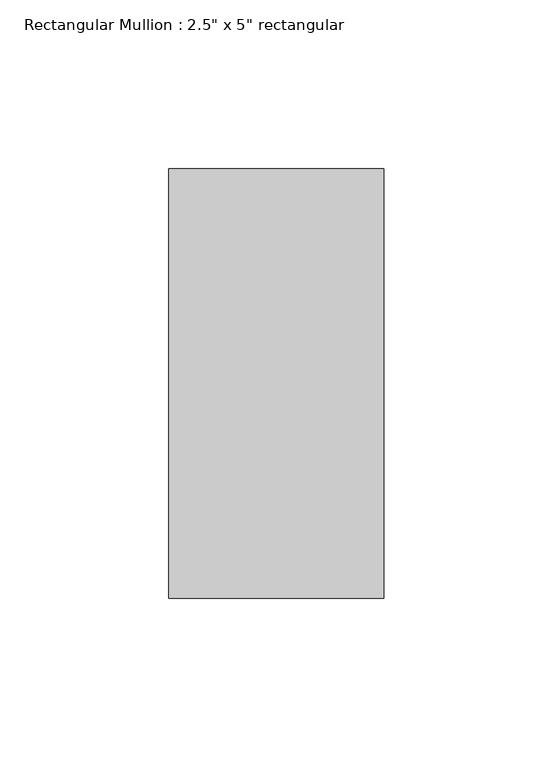
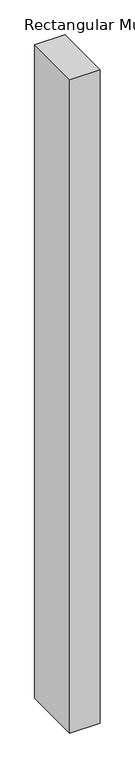
"""IFC4 building model written with IfcOpenShell, lengths in millimetres: member geometry."""

from ifc_helpers import new_model, si_unit, frame, origin, place, context, project, spatial, polyline, outline, extrude, source, transform, mapped, element, save


def member_f7b56663(model_context):
    return source(origin(), model_context, "Body", "SweptSolid", [
        extrude(outline(polyline([(31.75, 63.5), (31.75, -63.5), (-31.75, -63.5), (-31.75, 63.5), (31.75, 63.5)])), frame((0.0, 0.0, -1446.9815053), z_axis=(0.0, 0.0, 1.0), x_axis=(1.0, 0.0, 0.0)), (0.0, 0.0, 1.0), 1446.9815053),
    ])


if __name__ == "__main__":
    model = new_model("IFC4")
    model_context = context("Model", 3, world=origin())
    ifc_project = project(units=[si_unit("LENGTHUNIT", "METRE", prefix="MILLI")], contexts=[model_context])
    site = spatial("IfcSite", under=ifc_project)
    building = spatial("IfcBuilding", under=site)
    placement = place(None, origin())
    member_shape = member_f7b56663(model_context)
    element("IfcMember", 1, ObjectType="Rectangular Mullion : 2.5\" x 5\" rectangular", at=placement, inside=building, context=model_context, shape_type="MappedRepresentation", body=[
        mapped(member_shape, transform((0.0, 0.0, 0.0), x_axis=(1.0, 0.0, 0.0), y_axis=(0.0, 1.0, 0.0), z_axis=(0.0, 0.0, 1.0))),
    ])
    save(model, "model.ifc")

# Revit data of these elements
# Type "Rectangular Mullion : 2.5\" x 5\" rectangular"
#   built-in parameter 1007304 = 0.416667 (stored number, unit not read)
#   built-in parameter 1007301 = 0.104167 (stored number, unit not read)
#   built-in parameter 1007300 = 0.104167 (stored number, unit not read)
# Element 1 (IfcMember, "Rectangular Mullion : 2.5\" x 5\" rectangular")
#   Materials on its faces: "mullions"
# Materials
#   "mullions": class "Generic", colour RGB 120 120 120, transparency 0, Cost = 0
